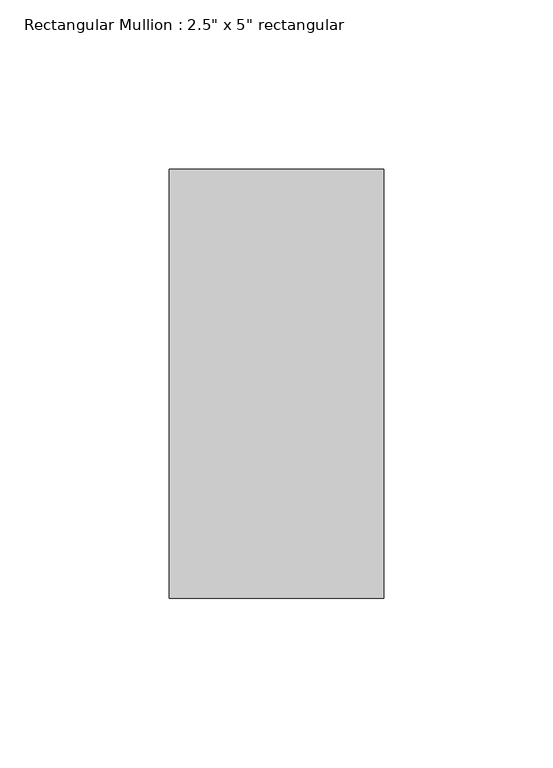
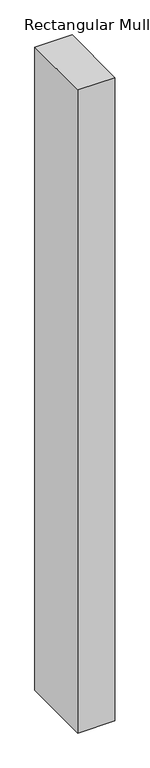
"""IFC4 building model written with IfcOpenShell, lengths in millimetres: member geometry."""

from ifc_helpers import new_model, si_unit, frame, origin, place, context, project, spatial, polyline, outline, extrude, source, transform, mapped, element, save


def member_2fc94954(model_context):
    return source(origin(), model_context, "Body", "SweptSolid", [
        extrude(outline(polyline([(0.0, 63.5), (0.0, -63.5), (-63.5, -63.5), (-63.5, 63.5), (0.0, 63.5)])), frame((0.0, 0.0, -1162.05), z_axis=(0.0, 0.0, 1.0), x_axis=(1.0, 0.0, 0.0)), (0.0, 0.0, 1.0), 1162.05),
    ])


if __name__ == "__main__":
    model = new_model("IFC4")
    model_context = context("Model", 3, world=origin())
    ifc_project = project(units=[si_unit("LENGTHUNIT", "METRE", prefix="MILLI")], contexts=[model_context])
    site = spatial("IfcSite", under=ifc_project)
    building = spatial("IfcBuilding", under=site)
    placement = place(None, origin())
    member_shape = member_2fc94954(model_context)
    element("IfcMember", 1, ObjectType="Rectangular Mullion : 2.5\" x 5\" rectangular", at=placement, inside=building, context=model_context, shape_type="MappedRepresentation", body=[
        mapped(member_shape, transform((0.0, 0.0, 0.0), x_axis=(1.0, 0.0, 0.0), y_axis=(0.0, 1.0, 0.0), z_axis=(0.0, 0.0, 1.0))),
    ])
    save(model, "model.ifc")

# Revit data of these elements
# Type "Rectangular Mullion : 2.5\" x 5\" rectangular"
#   built-in parameter 1007304 = 0.416667 (stored number, unit not read)
#   built-in parameter 1007301 = 0.104167 (stored number, unit not read)
#   built-in parameter 1007300 = 0.104167 (stored number, unit not read)
